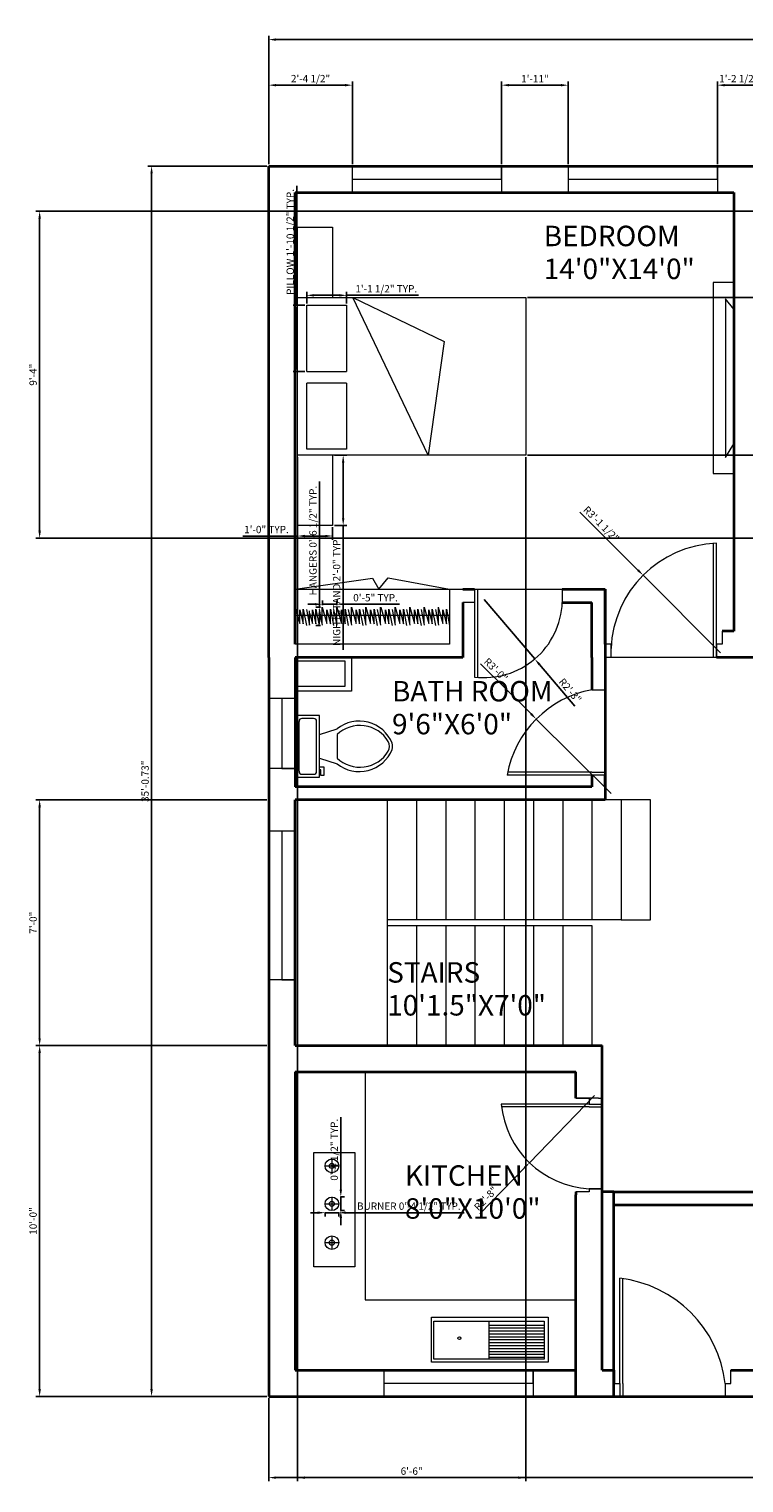
# Model space of a CAD drawing. Units: inches. Extents: x 1379 to 1989, y 1900 to 2397.
# Tile 1 of 3: x 1379 to 1623, y 1900 to 2397. Entities that reach past the tile are written whole.
import ezdxf

# ---------------------------------------------------------------- set-up
doc = ezdxf.new("R2010")
doc.units = ezdxf.units.IN
for name, color, linetype, lineweight in [('A-ANNO-DIMS', 2, 'Continuous', 18), ('A-AREA-IDEN', 7, 'Continuous', 18), ('A-DOOR', 3, 'Continuous', 18), ('A-EQPM', 9, 'Continuous', 18), ('A-FLOR-CASE', 9, 'Continuous', 18), ('A-FLOR-FIXT', 8, 'Continuous', 18), ('A-FLOR-FIXT-PATT', 8, 'Continuous', 13), ('A-FLOR-STRS', 7, 'Continuous', 18), ('A-FURN', 8, 'Continuous', 18), ('A-GLAZ', 4, 'Continuous', 18), ('A-WALL', 7, 'Continuous', 35)]:
    doc.layers.add(name, color=color, linetype=linetype, lineweight=lineweight)
doc.styles.get("Standard").update_dxf_attribs({"font": 'arial.ttf'})
doc.dimstyles.new('ISO-25', dxfattribs={"dimtxt": 2.5, "dimasz": 2.5, "dimexe": 1.25, "dimexo": 0.625, "dimtad": 1, "dimlunit": 3, "dimtxsty": 'Standard', "dimcen": 2.5, "dimadec": 0, "dimazin": 0, "dimtfac": 1, "dimtmove": 0, "dimatfit": 3, "dimfxl": 1, "dimarcsym": 0})

# ---------------------------------------------------------------- blocks, each defined once
blk = doc.blocks.new('*U2')
for p, q in [((9.5, -6), (9.5, -2)), ((-10, -8.5), (-8, -8.5)), ((-10, -9.5), (-10, -8.5)), ((-7, -9.5), (-10, -9.5)), ((-8, -8.5), (-8, -8)), ((-7, -8), (-7, -9.5)), ((-4, -8), (-6, -14)), ((4, -8), (6, -14)), ((4, -14), (-4, -14))]:
    blk.add_line(p, q)
blk.add_lwpolyline([(10.5, -8), (10.5, 0), (-10.5, 0), (-10.5, -8)], close=True)
for points in [[(-9.5, -2), (-9.5, -6)], [(8.5, -1), (-8.5, -1)], [(-8.5, -7), (8.5, -7)]]:
    blk.add_lwpolyline(points)
for centre, radius, start, end in [((-8.62, -1.88), 0.884, 81.8699, 188.1301), ((8.62, -1.88), 0.884, 351.8699, 98.1301), ((-8.62, -6.12), 0.884, 171.8699, 278.1301), ((8.62, -6.12), 0.884, 261.8699, 8.1301), ((3.52, -21.58), 12.17, 141.4691, 247.9714), ((4.2, -21.82), 11.33, 136.3677, 238.9468), ((-3.52, -21.58), 12.17, 292.0284, 38.5307), ((-4.2, -21.82), 11.33, 301.053, 43.6321), ((0, -27.88), 4, 245.7318, 294.2682), ((0, -29), 4, 254.8605, 285.1395)]:
    blk.add_arc(centre, radius, start, end)
blk = doc.blocks.new('*D6')
at = {"layer": 'A-ANNO-DIMS', "color": 0, "lineweight": -2, "transparency": 16777216}
for p, q in [((1460.41, 2350.93), (1460.41, 2394.79)), ((1462.91, 2393.54), (1912.41, 2393.54)), ((1914.91, 2350.93), (1914.91, 2394.79))]:
    blk.add_line(p, q, dxfattribs=at)
at = {"layer": 'A-ANNO-DIMS', "color": 0, "transparency": 16777216}
for points in [[(1462.91, 2393.95), (1462.91, 2393.12), (1460.41, 2393.54)], [(1912.41, 2393.95), (1912.41, 2393.12), (1914.91, 2393.54)]]:
    blk.add_solid(points, dxfattribs=at)
at = {"layer": 'Defpoints', "color": 0, "transparency": 16777216}
for p in [(1914.91, 2393.54), (1460.41, 2350.31), (1914.91, 2350.31)]:
    blk.add_point(p, dxfattribs=at)
at = {"layer": 'A-ANNO-DIMS', "color": 0, "transparency": 16777216, "insert": (1687.66, 2395.44), "char_height": 2.5, "attachment_point": 5}
blk.add_mtext('37\'-10.5"', dxfattribs=at)
blk = doc.blocks.new('*D7')
at = {"layer": 'A-ANNO-DIMS', "color": 0, "lineweight": -2, "transparency": 16777216}
for p, q in [((1459.79, 2350.31), (1419.13, 2350.31)), ((1420.38, 2347.81), (1420.38, 1932.08)), ((1459.79, 1929.58), (1419.13, 1929.58))]:
    blk.add_line(p, q, dxfattribs=at)
at = {"layer": 'A-ANNO-DIMS', "color": 0, "transparency": 16777216}
for points in [[(1419.96, 2347.81), (1420.79, 2347.81), (1420.38, 2350.31)], [(1419.96, 1932.08), (1420.79, 1932.08), (1420.38, 1929.58)]]:
    blk.add_solid(points, dxfattribs=at)
at = {"layer": 'Defpoints', "color": 0, "transparency": 16777216}
for p in [(1460.41, 2350.31), (1420.38, 1929.58), (1460.41, 1929.58)]:
    blk.add_point(p, dxfattribs=at)
at = {"layer": 'A-ANNO-DIMS', "color": 0, "transparency": 16777216, "insert": (1418.48, 2139.94), "char_height": 2.5, "attachment_point": 5, "rotation": 90}
blk.add_mtext('35\'-0.73"', dxfattribs=at)
blk = doc.blocks.new('WIN-51IN')
for p, q in [((0, 51), (9, 51)), ((4.5, 51), (4.5, 0)), ((9, 0), (0, 0)), ((4.5, 0), (9, 0))]:
    blk.add_line(p, q)
blk = doc.blocks.new('WIN-24IN')
for p, q in [((0, 24), (9, 24)), ((4.5, 24), (4.5, 0)), ((9, 0), (0, 0)), ((4.5, 0), (9, 0))]:
    blk.add_line(p, q)
blk = doc.blocks.new('COOKTOP-BURNER')
for p, q in [((0, 2.33), (4.67, 2.33)), ((2.33, 4.67), (2.33, 0))]:
    blk.add_line(p, q)
for radius in [2.33, 0.875]:
    blk.add_circle((2.33, 2.33), radius)
blk = doc.blocks.new('BED-PILLOW')
blk.add_line((0, 0), (13.66, 0))
blk.add_lwpolyline([(0, 0), (0, 22.6), (13.66, 22.6), (13.66, 0)])
blk = doc.blocks.new('CLOSET-GARMENT-CLUSTER')
for p, q in [((0, 6.34), (1.58, 0.7)), ((1.58, 0.7), (1.58, 5.41)), ((1.58, 5.41), (2.79, 0.56)), ((2.79, 0.56), (2.79, 5.59)), ((2.79, 5.59), (3.87, 0)), ((3.87, 5.45), (4.94, 0.19)), ((4.94, 0.83), (4.94, 6.28))]:
    blk.add_line(p, q)
blk = doc.blocks.new('CLOSET-GARMENT-CLUSTER-END')
for p, q in [((0, 5.45), (1.07, 0.19)), ((1.07, 0.19), (1.07, 5.08)), ((2.05, 0.7), (2.05, 5.41)), ((2.05, 5.41), (3.26, 0.56)), ((3.26, 0.56), (3.26, 5.59)), ((3.26, 5.59), (4.34, 0)), ((4.34, 5.45), (5.41, 0.19)), ((5.41, 0.83), (5.41, 6.28)), ((1.07, 0.83), (1.07, 4.19)), ((1.07, 4.19), (2.05, 0.7))]:
    blk.add_line(p, q)
blk = doc.blocks.new('BEDSIDE-TABLE-12X24')
for p, q in [((0, 0), (0, 24)), ((0, 24), (12, 24)), ((12, 24), (12, 0))]:
    blk.add_line(p, q)
blk = doc.blocks.new('*D19')
at = {"layer": 'A-ANNO-DIMS', "color": 0, "lineweight": -2, "transparency": 16777216}
for p, q in [((1470, 2302.71), (1470, 2343.51)), ((1472.76, 2302.71), (1468.75, 2302.71)), ((1470, 2282.61), (1470, 2300.21)), ((1472.76, 2280.11), (1468.75, 2280.11))]:
    blk.add_line(p, q, dxfattribs=at)
at = {"layer": 'A-ANNO-DIMS', "color": 0, "transparency": 16777216}
for points in [[(1469.58, 2300.21), (1470.42, 2300.21), (1470, 2302.71)], [(1469.58, 2282.61), (1470.42, 2282.61), (1470, 2280.11)]]:
    blk.add_solid(points, dxfattribs=at)
at = {"layer": 'Defpoints', "color": 0, "transparency": 16777216}
for p in [(1470, 2302.71), (1473.39, 2302.71), (1473.39, 2280.11)]:
    blk.add_point(p, dxfattribs=at)
at = {"layer": 'A-ANNO-DIMS', "color": 0, "transparency": 16777216, "insert": (1468.08, 2324.36), "char_height": 2.5, "attachment_point": 5, "rotation": 90}
blk.add_mtext('PILLOW 1\'-10 1/2" TYP.', dxfattribs=at)
blk = doc.blocks.new('*D20')
at = {"layer": 'A-ANNO-DIMS', "color": 0, "lineweight": -2, "transparency": 16777216}
for p, q in [((1473.39, 2303.34), (1473.39, 2307.35)), ((1487.05, 2303.34), (1487.05, 2307.35)), ((1475.89, 2306.1), (1484.55, 2306.1)), ((1487.05, 2306.1), (1511.63, 2306.1))]:
    blk.add_line(p, q, dxfattribs=at)
at = {"layer": 'A-ANNO-DIMS', "color": 0, "transparency": 16777216}
for points in [[(1475.89, 2306.52), (1475.89, 2305.68), (1473.39, 2306.1)], [(1484.55, 2306.52), (1484.55, 2305.68), (1487.05, 2306.1)]]:
    blk.add_solid(points, dxfattribs=at)
at = {"layer": 'Defpoints', "color": 0, "transparency": 16777216}
for p in [(1473.39, 2302.71), (1487.05, 2306.1), (1487.05, 2302.71)]:
    blk.add_point(p, dxfattribs=at)
at = {"layer": 'A-ANNO-DIMS', "color": 0, "transparency": 16777216, "insert": (1500.59, 2308.02), "char_height": 2.5, "attachment_point": 5}
blk.add_mtext('1\'-1 1/2" TYP.', dxfattribs=at)
blk = doc.blocks.new('*D21')
at = {"layer": 'A-ANNO-DIMS', "color": 0, "lineweight": -2, "transparency": 16777216}
for p, q in [((1482.89, 2251.4), (1487.12, 2251.4)), ((1485.87, 2248.9), (1485.87, 2229.9)), ((1482.89, 2227.4), (1487.12, 2227.4)), ((1485.87, 2227.4), (1485.87, 2184.86))]:
    blk.add_line(p, q, dxfattribs=at)
at = {"layer": 'A-ANNO-DIMS', "color": 0, "transparency": 16777216}
for points in [[(1485.45, 2248.9), (1486.28, 2248.9), (1485.87, 2251.4)], [(1485.45, 2229.9), (1486.28, 2229.9), (1485.87, 2227.4)]]:
    blk.add_solid(points, dxfattribs=at)
at = {"layer": 'Defpoints', "color": 0, "transparency": 16777216}
for p in [(1482.27, 2251.4), (1482.27, 2227.4), (1485.87, 2227.4)]:
    blk.add_point(p, dxfattribs=at)
at = {"layer": 'A-ANNO-DIMS', "color": 0, "transparency": 16777216, "insert": (1483.95, 2204.88), "char_height": 2.5, "attachment_point": 5, "rotation": 90}
blk.add_mtext('NIGHTSTAND 2\'-0" TYP.', dxfattribs=at)
blk = doc.blocks.new('*D22')
at = {"layer": 'A-ANNO-DIMS', "color": 0, "lineweight": -2, "transparency": 16777216}
for p, q in [((1470.27, 2223.8), (1451.51, 2223.8)), ((1470.27, 2226.77), (1470.27, 2222.55)), ((1479.77, 2223.8), (1472.77, 2223.8)), ((1482.27, 2226.77), (1482.27, 2222.55))]:
    blk.add_line(p, q, dxfattribs=at)
at = {"layer": 'A-ANNO-DIMS', "color": 0, "transparency": 16777216}
for points in [[(1472.77, 2224.21), (1472.77, 2223.38), (1470.27, 2223.8)], [(1479.77, 2224.21), (1479.77, 2223.38), (1482.27, 2223.8)]]:
    blk.add_solid(points, dxfattribs=at)
at = {"layer": 'Defpoints', "color": 0, "transparency": 16777216}
for p in [(1470.27, 2227.4), (1482.27, 2227.4), (1470.27, 2223.8)]:
    blk.add_point(p, dxfattribs=at)
at = {"layer": 'A-ANNO-DIMS', "color": 0, "transparency": 16777216, "insert": (1459.64, 2225.7), "char_height": 2.5, "attachment_point": 5}
blk.add_mtext('1\'-0" TYP.', dxfattribs=at)
blk = doc.blocks.new('*D23')
at = {"layer": 'A-ANNO-DIMS', "color": 0, "lineweight": -2, "transparency": 16777216}
for p, q in [((1477.19, 1992.42), (1474.69, 1992.42)), ((1479.69, 1992.5), (1479.69, 1991.17)), ((1479.69, 1992.42), (1484.35, 1992.42)), ((1484.35, 1992.5), (1484.35, 1991.17)), ((1486.85, 1992.42), (1527.27, 1992.42))]:
    blk.add_line(p, q, dxfattribs=at)
at = {"layer": 'A-ANNO-DIMS', "color": 0, "transparency": 16777216}
for points in [[(1477.19, 1992.84), (1477.19, 1992), (1479.69, 1992.42)], [(1486.85, 1992.84), (1486.85, 1992), (1484.35, 1992.42)]]:
    blk.add_solid(points, dxfattribs=at)
at = {"layer": 'Defpoints', "color": 0, "transparency": 16777216}
for p in [(1479.69, 1993.12), (1484.35, 1993.12), (1484.35, 1992.42)]:
    blk.add_point(p, dxfattribs=at)
at = {"layer": 'A-ANNO-DIMS', "color": 0, "transparency": 16777216, "insert": (1508.31, 1994.34), "char_height": 2.5, "attachment_point": 5}
blk.add_mtext('BURNER 0\'-4 1/2" TYP.', dxfattribs=at)
blk = doc.blocks.new('*D24')
at = {"layer": 'A-ANNO-DIMS', "color": 0, "lineweight": -2, "transparency": 16777216}
for p, q in [((1485.05, 2000.29), (1485.05, 2025.1)), ((1484.98, 1997.79), (1486.3, 1997.79)), ((1485.05, 1993.12), (1485.05, 1997.79)), ((1484.98, 1993.12), (1486.3, 1993.12)), ((1485.05, 1990.62), (1485.05, 1988.12))]:
    blk.add_line(p, q, dxfattribs=at)
at = {"layer": 'A-ANNO-DIMS', "color": 0, "transparency": 16777216}
for points in [[(1484.64, 2000.29), (1485.47, 2000.29), (1485.05, 1997.79)], [(1484.64, 1990.62), (1485.47, 1990.62), (1485.05, 1993.12)]]:
    blk.add_solid(points, dxfattribs=at)
at = {"layer": 'Defpoints', "color": 0, "transparency": 16777216}
for p in [(1484.35, 1997.79), (1485.05, 1997.79), (1484.35, 1993.12)]:
    blk.add_point(p, dxfattribs=at)
at = {"layer": 'A-ANNO-DIMS', "color": 0, "transparency": 16777216, "insert": (1483.14, 2013.94), "char_height": 2.5, "attachment_point": 5, "rotation": 90}
blk.add_mtext('0\'-4 1/2" TYP.', dxfattribs=at)
blk = doc.blocks.new('*D25')
at = {"layer": 'A-ANNO-DIMS', "color": 0, "lineweight": -2, "transparency": 16777216}
for p, q in [((1477.79, 2199.52), (1477.79, 2242.44)), ((1478.11, 2199.52), (1476.54, 2199.52)), ((1478.11, 2193.18), (1476.54, 2193.18)), ((1477.79, 2195.68), (1477.79, 2197.02))]:
    blk.add_line(p, q, dxfattribs=at)
at = {"layer": 'A-ANNO-DIMS', "color": 0, "transparency": 16777216}
for points in [[(1477.37, 2197.02), (1478.2, 2197.02), (1477.79, 2199.52)], [(1477.37, 2195.68), (1478.2, 2195.68), (1477.79, 2193.18)]]:
    blk.add_solid(points, dxfattribs=at)
at = {"layer": 'Defpoints', "color": 0, "transparency": 16777216}
for p in [(1477.79, 2199.52), (1478.74, 2199.52), (1478.74, 2193.18)]:
    blk.add_point(p, dxfattribs=at)
at = {"layer": 'A-ANNO-DIMS', "color": 0, "transparency": 16777216, "insert": (1475.87, 2222.23), "char_height": 2.5, "attachment_point": 5, "rotation": 90}
blk.add_mtext('HANGERS 0\'-6 1/2" TYP.', dxfattribs=at)
blk = doc.blocks.new('*D26')
at = {"layer": 'A-ANNO-DIMS', "color": 0, "lineweight": -2, "transparency": 16777216}
for p, q in [((1476.24, 2200.47), (1473.74, 2200.47)), ((1478.74, 2200.14), (1478.74, 2201.72)), ((1478.74, 2200.47), (1483.68, 2200.47)), ((1483.68, 2200.14), (1483.68, 2201.72)), ((1486.18, 2200.47), (1505.17, 2200.47))]:
    blk.add_line(p, q, dxfattribs=at)
at = {"layer": 'A-ANNO-DIMS', "color": 0, "transparency": 16777216}
for points in [[(1476.24, 2200.88), (1476.24, 2200.05), (1478.74, 2200.47)], [(1486.18, 2200.88), (1486.18, 2200.05), (1483.68, 2200.47)]]:
    blk.add_solid(points, dxfattribs=at)
at = {"layer": 'Defpoints', "color": 0, "transparency": 16777216}
for p in [(1478.74, 2199.52), (1483.68, 2200.47), (1483.68, 2199.52)]:
    blk.add_point(p, dxfattribs=at)
at = {"layer": 'A-ANNO-DIMS', "color": 0, "transparency": 16777216, "insert": (1496.92, 2202.37), "char_height": 2.5, "attachment_point": 5}
blk.add_mtext('0\'-5" TYP.', dxfattribs=at)
blk = doc.blocks.new('*D29')
at = {"layer": 'A-ANNO-DIMS', "color": 0, "lineweight": -2, "transparency": 16777216}
for p, q in [((1959.91, 1941.48), (1959.91, 1900.58)), ((1460.41, 1928.96), (1460.41, 1900.58)), ((1462.91, 1901.83), (1957.41, 1901.83))]:
    blk.add_line(p, q, dxfattribs=at)
at = {"layer": 'A-ANNO-DIMS', "color": 0, "transparency": 16777216}
for points in [[(1462.91, 1902.24), (1462.91, 1901.41), (1460.41, 1901.83)], [(1957.41, 1902.24), (1957.41, 1901.41), (1959.91, 1901.83)]]:
    blk.add_solid(points, dxfattribs=at)
at = {"layer": 'Defpoints', "color": 0, "transparency": 16777216}
for p in [(1959.91, 1942.11), (1460.41, 1929.58), (1959.91, 1901.83)]:
    blk.add_point(p, dxfattribs=at)
at = {"layer": 'A-ANNO-DIMS', "color": 0, "transparency": 16777216, "insert": (1710.16, 1903.75), "char_height": 2.5, "attachment_point": 5}
blk.add_mtext('41\'-7 1/2"', dxfattribs=at)
blk = doc.blocks.new('*D33')
at = {"layer": 'A-ANNO-DIMS', "color": 0, "lineweight": -2, "transparency": 16777216}
for p, q in [((1460.41, 2350.93), (1460.41, 2379.21)), ((1462.91, 2377.96), (1486.52, 2377.96)), ((1489.02, 2350.93), (1489.02, 2379.21))]:
    blk.add_line(p, q, dxfattribs=at)
at = {"layer": 'A-ANNO-DIMS', "color": 0, "transparency": 16777216}
for points in [[(1462.91, 2378.37), (1462.91, 2377.54), (1460.41, 2377.96)], [(1486.52, 2378.37), (1486.52, 2377.54), (1489.02, 2377.96)]]:
    blk.add_solid(points, dxfattribs=at)
at = {"layer": 'Defpoints', "color": 0, "transparency": 16777216}
for p in [(1489.02, 2377.96), (1460.41, 2350.31), (1489.02, 2350.31)]:
    blk.add_point(p, dxfattribs=at)
at = {"layer": 'A-ANNO-DIMS', "color": 0, "transparency": 16777216, "insert": (1474.71, 2379.88), "char_height": 2.5, "attachment_point": 5}
blk.add_mtext('2\'-4 1/2"', dxfattribs=at)
blk = doc.blocks.new('*D34')
at = {"layer": 'A-ANNO-DIMS', "color": 0, "lineweight": -2, "transparency": 16777216}
for p, q in [((1540.02, 2350.93), (1540.02, 2379.21)), ((1542.52, 2377.96), (1560.28, 2377.96)), ((1562.78, 2350.93), (1562.78, 2379.21))]:
    blk.add_line(p, q, dxfattribs=at)
at = {"layer": 'A-ANNO-DIMS', "color": 0, "transparency": 16777216}
for points in [[(1542.52, 2378.37), (1542.52, 2377.54), (1540.02, 2377.96)], [(1560.28, 2378.37), (1560.28, 2377.54), (1562.78, 2377.96)]]:
    blk.add_solid(points, dxfattribs=at)
at = {"layer": 'Defpoints', "color": 0, "transparency": 16777216}
for p in [(1562.78, 2377.96), (1540.02, 2350.31), (1562.78, 2350.31)]:
    blk.add_point(p, dxfattribs=at)
at = {"layer": 'A-ANNO-DIMS', "color": 0, "transparency": 16777216, "insert": (1551.4, 2379.84), "char_height": 2.5, "attachment_point": 5}
blk.add_mtext('1\'-11"', dxfattribs=at)
blk = doc.blocks.new('*D35')
at = {"layer": 'A-ANNO-DIMS', "color": 0, "lineweight": -2, "transparency": 16777216}
for p, q in [((1613.78, 2350.93), (1613.78, 2379.21)), ((1616.28, 2377.96), (1625.91, 2377.96)), ((1628.41, 2350.93), (1628.41, 2379.21))]:
    blk.add_line(p, q, dxfattribs=at)
at = {"layer": 'A-ANNO-DIMS', "color": 0, "transparency": 16777216}
for points in [[(1616.28, 2378.37), (1616.28, 2377.54), (1613.78, 2377.96)], [(1625.91, 2378.37), (1625.91, 2377.54), (1628.41, 2377.96)]]:
    blk.add_solid(points, dxfattribs=at)
at = {"layer": 'Defpoints', "color": 0, "transparency": 16777216}
for p in [(1628.41, 2377.96), (1613.78, 2350.31), (1628.41, 2350.31)]:
    blk.add_point(p, dxfattribs=at)
at = {"layer": 'A-ANNO-DIMS', "color": 0, "transparency": 16777216, "insert": (1621.1, 2379.88), "char_height": 2.5, "attachment_point": 5}
blk.add_mtext('1\'-2 1/2"', dxfattribs=at)
blk = doc.blocks.new('*D38')
at = {"layer": 'A-ANNO-DIMS', "color": 0, "lineweight": -2, "transparency": 16777216}
for p, q in [((1459.79, 2049.58), (1380.86, 2049.58)), ((1382.11, 1932.08), (1382.11, 2047.08)), ((1459.79, 1929.58), (1380.86, 1929.58))]:
    blk.add_line(p, q, dxfattribs=at)
at = {"layer": 'A-ANNO-DIMS', "color": 0, "transparency": 16777216}
for points in [[(1381.7, 2047.08), (1382.53, 2047.08), (1382.11, 2049.58)], [(1381.7, 1932.08), (1382.53, 1932.08), (1382.11, 1929.58)]]:
    blk.add_solid(points, dxfattribs=at)
at = {"layer": 'Defpoints', "color": 0, "transparency": 16777216}
for p in [(1382.11, 2049.58), (1460.41, 2049.58), (1460.41, 1929.58)]:
    blk.add_point(p, dxfattribs=at)
at = {"layer": 'A-ANNO-DIMS', "color": 0, "transparency": 16777216, "insert": (1380.21, 1989.58), "char_height": 2.5, "attachment_point": 5, "rotation": 90}
blk.add_mtext('10\'-0"', dxfattribs=at)
blk = doc.blocks.new('*D39')
at = {"layer": 'A-ANNO-DIMS', "color": 0, "lineweight": -2, "transparency": 16777216}
for p, q in [((1459.79, 2133.58), (1380.86, 2133.58)), ((1382.11, 2052.08), (1382.11, 2131.08)), ((1459.79, 2049.58), (1380.86, 2049.58))]:
    blk.add_line(p, q, dxfattribs=at)
at = {"layer": 'A-ANNO-DIMS', "color": 0, "transparency": 16777216}
for points in [[(1381.7, 2131.08), (1382.53, 2131.08), (1382.11, 2133.58)], [(1381.7, 2052.08), (1382.53, 2052.08), (1382.11, 2049.58)]]:
    blk.add_solid(points, dxfattribs=at)
at = {"layer": 'Defpoints', "color": 0, "transparency": 16777216}
for p in [(1382.11, 2133.58), (1460.41, 2133.58), (1460.41, 2049.58)]:
    blk.add_point(p, dxfattribs=at)
at = {"layer": 'A-ANNO-DIMS', "color": 0, "transparency": 16777216, "insert": (1380.21, 2091.58), "char_height": 2.5, "attachment_point": 5, "rotation": 90}
blk.add_mtext('7\'-0"', dxfattribs=at)
blk = doc.blocks.new('*D40')
at = {"layer": 'A-ANNO-DIMS', "color": 0, "lineweight": -2, "transparency": 16777216}
for p, q in [((1470.27, 2250.77), (1470.27, 1900.58)), ((1548.27, 2250.77), (1548.27, 1900.58)), ((1472.77, 1901.83), (1545.77, 1901.83))]:
    blk.add_line(p, q, dxfattribs=at)
at = {"layer": 'A-ANNO-DIMS', "color": 0, "transparency": 16777216}
for points in [[(1472.77, 1902.24), (1472.77, 1901.41), (1470.27, 1901.83)], [(1545.77, 1902.24), (1545.77, 1901.41), (1548.27, 1901.83)]]:
    blk.add_solid(points, dxfattribs=at)
at = {"layer": 'Defpoints', "color": 0, "transparency": 16777216}
for p in [(1470.27, 2251.4), (1548.27, 2251.4), (1548.27, 1901.83)]:
    blk.add_point(p, dxfattribs=at)
at = {"layer": 'A-ANNO-DIMS', "color": 0, "transparency": 16777216, "insert": (1509.27, 1903.73), "char_height": 2.5, "attachment_point": 5}
blk.add_mtext('6\'-6"', dxfattribs=at)
blk = doc.blocks.new('*D41')
at = {"layer": 'A-ANNO-DIMS', "color": 0, "lineweight": -2, "transparency": 16777216}
for p, q in [((1548.89, 2305.4), (1988.81, 2305.4)), ((1987.56, 2302.9), (1987.56, 2253.9)), ((1548.89, 2251.4), (1988.81, 2251.4))]:
    blk.add_line(p, q, dxfattribs=at)
at = {"layer": 'A-ANNO-DIMS', "color": 0, "transparency": 16777216}
for points in [[(1987.14, 2302.9), (1987.98, 2302.9), (1987.56, 2305.4)], [(1987.14, 2253.9), (1987.98, 2253.9), (1987.56, 2251.4)]]:
    blk.add_solid(points, dxfattribs=at)
at = {"layer": 'Defpoints', "color": 0, "transparency": 16777216}
for p in [(1548.27, 2305.4), (1548.27, 2251.4), (1987.56, 2251.4)]:
    blk.add_point(p, dxfattribs=at)
at = {"layer": 'A-ANNO-DIMS', "color": 0, "transparency": 16777216, "insert": (1985.66, 2278.4), "char_height": 2.5, "attachment_point": 5, "rotation": 90}
blk.add_mtext('4\'-6"', dxfattribs=at)
blk = doc.blocks.new('*D43')
at = {"layer": 'A-ANNO-DIMS', "color": 0, "lineweight": -2, "transparency": 16777216}
for p, q in [((1811.35, 2334.84), (1380.86, 2334.84)), ((1382.11, 2332.34), (1382.11, 2225.59)), ((1875.73, 2223.09), (1380.86, 2223.09))]:
    blk.add_line(p, q, dxfattribs=at)
at = {"layer": 'A-ANNO-DIMS', "color": 0, "transparency": 16777216}
for points in [[(1381.7, 2332.34), (1382.53, 2332.34), (1382.11, 2334.84)], [(1381.7, 2225.59), (1382.53, 2225.59), (1382.11, 2223.09)]]:
    blk.add_solid(points, dxfattribs=at)
at = {"layer": 'Defpoints', "color": 0, "transparency": 16777216}
for p in [(1811.97, 2334.84), (1382.11, 2223.09), (1876.36, 2223.09)]:
    blk.add_point(p, dxfattribs=at)
at = {"layer": 'A-ANNO-DIMS', "color": 0, "transparency": 16777216, "insert": (1380.21, 2278.96), "char_height": 2.5, "attachment_point": 5, "rotation": 90}
blk.add_mtext('9\'-4"', dxfattribs=at)
blk = doc.blocks.new('*D46')
at = {"layer": 'A-ANNO-DIMS', "color": 0, "lineweight": -2, "transparency": 16777216}
for p, q in [((1566.8, 2232), (1586.62, 2212.15)), ((1614.88, 2183.84), (1588.38, 2210.38))]:
    blk.add_line(p, q, dxfattribs=at)
at = {"layer": 'A-ANNO-DIMS', "color": 0, "transparency": 16777216}
blk.add_solid([(1586.91, 2212.44), (1586.32, 2211.85), (1588.38, 2210.38)], dxfattribs=at)
at = {"layer": 'Defpoints', "color": 0, "transparency": 16777216}
for p in [(1588.38, 2210.38), (1614.88, 2183.84)]:
    blk.add_point(p, dxfattribs=at)
at = {"layer": 'A-ANNO-DIMS', "color": 0, "transparency": 16777216, "insert": (1573.85, 2227.65), "char_height": 2.5, "attachment_point": 5, "rotation": 314.9518}
blk.add_mtext('R3\'-1 1/2"', dxfattribs=at)
blk = doc.blocks.new('*D47')
at = {"layer": 'A-ANNO-DIMS', "color": 0, "lineweight": -2, "transparency": 16777216}
for p, q in [((1532.83, 2180.11), (1550.08, 2162.96)), ((1577.48, 2135.72), (1551.85, 2161.2))]:
    blk.add_line(p, q, dxfattribs=at)
at = {"layer": 'A-ANNO-DIMS', "color": 0, "transparency": 16777216}
blk.add_solid([(1550.37, 2163.26), (1549.79, 2162.67), (1551.85, 2161.2)], dxfattribs=at)
at = {"layer": 'Defpoints', "color": 0, "transparency": 16777216}
for p in [(1551.85, 2161.2), (1577.48, 2135.72)]:
    blk.add_point(p, dxfattribs=at)
at = {"layer": 'A-ANNO-DIMS', "color": 0, "transparency": 16777216, "insert": (1537.82, 2177.83), "char_height": 2.5, "attachment_point": 5, "rotation": 315.173}
blk.add_mtext('R3\'-0"', dxfattribs=at)
blk = doc.blocks.new('*D48')
at = {"layer": 'A-ANNO-DIMS', "color": 0, "lineweight": -2, "transparency": 16777216}
for p, q in [((1571.77, 2032.52), (1549.53, 2009.52)), ((1532.61, 1992.02), (1547.79, 2007.72))]:
    blk.add_line(p, q, dxfattribs=at)
at = {"layer": 'A-ANNO-DIMS', "color": 0, "transparency": 16777216}
blk.add_solid([(1547.5, 2008.01), (1548.09, 2007.43), (1549.53, 2009.52)], dxfattribs=at)
at = {"layer": 'Defpoints', "color": 0, "transparency": 16777216}
for p in [(1571.77, 2032.52), (1549.53, 2009.52)]:
    blk.add_point(p, dxfattribs=at)
at = {"layer": 'A-ANNO-DIMS', "color": 0, "transparency": 16777216, "insert": (1534.82, 1997.04), "char_height": 2.5, "attachment_point": 5, "rotation": 45.9708}
blk.add_mtext('R2\'-8"', dxfattribs=at)
blk = doc.blocks.new('*D49')
at = {"layer": 'A-ANNO-DIMS', "color": 0, "lineweight": -2, "transparency": 16777216}
for p, q in [((1534.02, 2202.14), (1551.35, 2181.75)), ((1565.08, 2165.6), (1552.97, 2179.85))]:
    blk.add_line(p, q, dxfattribs=at)
at = {"layer": 'A-ANNO-DIMS', "color": 0, "transparency": 16777216}
blk.add_solid([(1553.28, 2180.12), (1552.65, 2179.58), (1551.35, 2181.75)], dxfattribs=at)
at = {"layer": 'Defpoints', "color": 0, "transparency": 16777216}
for p in [(1534.02, 2202.14), (1551.35, 2181.75)]:
    blk.add_point(p, dxfattribs=at)
at = {"layer": 'A-ANNO-DIMS', "color": 0, "transparency": 16777216, "insert": (1563.19, 2170.75), "char_height": 2.5, "attachment_point": 5, "rotation": 310.3656}
blk.add_mtext('R2\'-3"', dxfattribs=at)

msp = doc.modelspace()

# ---------------------------------------------------------------- hatches: boundary and pattern name
at = {"layer": 'A-FLOR-FIXT-PATT'}
h = msp.add_hatch(dxfattribs=at)
h.set_pattern_fill('ANSI31', color=256, scale=0.314961, angle=-45, style=0)
h.paths.add_polyline_path([(1535.728, 1942.741), (1554.59, 1942.741), (1554.59, 1954.741), (1535.728, 1954.741)])

# ---------------------------------------------------------------- linework, layer by layer
at = {"layer": 'A-DOOR'}
for p, q in [((1612.41, 2185.308), (1612.41, 2221.255)), ((1613.41, 2185.308), (1613.41, 2221.308)), ((1530.753, 2205.582), (1530.753, 2201.082)), ((1530.753, 2205.582), (1560.753, 2205.582)), ((1530.753, 2205.582), (1530.753, 2175.582)), ((1531.753, 2205.582), (1531.753, 2175.582)), ((1560.753, 2205.582), (1560.753, 2201.082)), ((1530.753, 2201.082), (1526.753, 2201.082)), ((1619.41, 2191.308), (1615.41, 2191.308)), ((1615.41, 2191.308), (1615.41, 2186.808)), ((1577.41, 2186.808), (1575.41, 2186.808)), ((1577.41, 2182.308), (1577.41, 2186.808)), ((1612.41, 2182.308), (1612.41, 2185.308)), ((1615.41, 2186.808), (1613.41, 2186.808)), ((1613.41, 2186.808), (1613.41, 2182.308)), ((1615.41, 2186.808), (1613.41, 2186.808)), ((1613.41, 2182.308), (1613.41, 2185.308)), ((1577.41, 2182.308), (1575.41, 2182.308)), ((1613.41, 2182.308), (1577.41, 2182.308)), ((1575.41, 2171.082), (1570.91, 2171.082)), ((1575.41, 2142.082), (1575.41, 2171.082)), ((1570.91, 2143.082), (1542.104, 2143.082)), ((1570.91, 2143.082), (1575.41, 2143.082)), ((1570.91, 2142.082), (1541.91, 2142.082)), ((1575.41, 2142.082), (1570.91, 2142.082)), ((1569.91, 2029.582), (1539.91, 2029.582)), ((1569.91, 2028.582), (1539.91, 2028.582)), ((1573.101, 2031.582), (1565.41, 2031.582)), ((1565.41, 2031.582), (1569.91, 2031.582)), ((1569.91, 2031.582), (1569.91, 2029.582)), ((1569.91, 2029.582), (1574.41, 2029.582)), ((1569.91, 2028.582), (1574.41, 2028.582)), ((1573.101, 2031.582), (1574.41, 2031.582)), ((1569.91, 1999.582), (1565.41, 1999.582)), ((1569.91, 2000.582), (1574.41, 2000.582)), ((1574.41, 2000.582), (1569.91, 2000.582)), ((1574.41, 2000.582), (1569.91, 2000.582)), ((1569.91, 2000.582), (1569.91, 1999.582)), ((1569.91, 1998.582), (1569.91, 1998.582)), ((1580.41, 1933.978), (1580.41, 1969.978)), ((1581.41, 1933.978), (1581.41, 1969.851)), ((1578.41, 1933.978), (1580.41, 1933.978)), ((1580.41, 1933.978), (1580.41, 1929.582)), ((1581.41, 1933.978), (1581.41, 1929.582)), ((1616.41, 1933.978), (1616.41, 1929.582)), ((1616.41, 1933.978), (1618.41, 1933.978)), ((1618.41, 1933.978), (1618.41, 1938.582))]:
    msp.add_line(p, q, dxfattribs=at)
for centre, radius, start, end in [((1614.877, 2183.838), 37.498, 92.24183, 177.66061), ((1534.019, 2202.136), 26.755, 262.98798, 357.7411), ((1577.485, 2135.723), 36.138, 100.48207, 169.86542), ((1571.769, 2032.522), 31.994, 185.27318, 266.66886), ((1575.755, 1929.322), 40.921, 6.53202, 83.46798)]:
    msp.add_arc(centre, radius, start, end, dxfattribs=at)
at = {"layer": 'A-EQPM'}
msp.add_lwpolyline([(1475.816, 2012.99), (1489.79, 2012.99), (1489.79, 1973.888), (1475.816, 1973.888)], close=True, dxfattribs=at)
at = {"layer": 'A-FLOR-CASE'}
for p, q in [((1469.41, 2205.582), (1495.864, 2209.393)), ((1495.864, 2209.393), (1498.082, 2205.582)), ((1498.082, 2205.582), (1501.217, 2209.468)), ((1501.217, 2209.468), (1522.253, 2205.582)), ((1469.41, 2205.582), (1526.753, 2205.582)), ((1522.253, 2205.582), (1522.253, 2186.808)), ((1469.41, 2199.516), (1470.993, 2193.877)), ((1470.993, 2193.877), (1470.993, 2198.584)), ((1470.993, 2198.584), (1472.205, 2193.737)), ((1472.205, 2193.737), (1472.205, 2198.77)), ((1472.205, 2198.77), (1473.278, 2193.178)), ((1518.339, 2199.516), (1519.921, 2193.877)), ((1519.921, 2193.877), (1519.921, 2198.584)), ((1519.921, 2198.584), (1521.134, 2193.737)), ((1521.134, 2193.737), (1521.134, 2198.77)), ((1521.134, 2198.77), (1522.206, 2193.178)), ((1522.206, 2198.63), (1522.253, 2198.401)), ((1469.41, 2196.735), (1522.253, 2196.735)), ((1522.253, 2186.808), (1469.41, 2186.808)), ((1469.41, 2040.582), (1493.41, 2040.582)), ((1493.41, 2040.582), (1493.41, 1962.582)), ((1469.41, 1938.582), (1469.41, 1962.582)), ((1493.41, 1962.582), (1565.41, 1962.582))]:
    msp.add_line(p, q, dxfattribs=at)
at = {"layer": 'A-FLOR-FIXT'}
for p, q in [((1469.41, 2181.084), (1486.48, 2181.084)), ((1486.48, 2182.308), (1488.751, 2182.308)), ((1486.48, 2181.084), (1486.48, 2172.322)), ((1488.751, 2182.308), (1488.751, 2170.738)), ((1486.48, 2172.322), (1469.41, 2172.322)), ((1535.728, 1942.369), (1535.728, 1955.283))]:
    msp.add_line(p, q, dxfattribs=at)
msp.add_lwpolyline([(1488.751, 2170.738), (1469.41, 2170.738)], dxfattribs=at)
for points in [[(1516.053, 1956.745), (1555.93, 1956.745), (1555.93, 1941.32), (1516.053, 1941.32)], [(1516.866, 1955.283), (1554.59, 1955.283), (1554.59, 1942.369), (1516.866, 1942.369)]]:
    msp.add_lwpolyline(points, close=True, dxfattribs=at)
msp.add_circle((1525.572, 1949.528), 0.499, dxfattribs=at)
at = {"layer": 'A-FLOR-STRS'}
for p, q in [((1500.91, 2133.582), (1500.91, 2092.582)), ((1510.91, 2133.582), (1510.91, 2092.582)), ((1520.91, 2133.582), (1520.91, 2092.582)), ((1530.91, 2133.582), (1530.91, 2092.582)), ((1540.91, 2133.582), (1540.91, 2092.582)), ((1550.91, 2133.582), (1550.91, 2092.582)), ((1560.91, 2133.582), (1560.91, 2092.582)), ((1590.91, 2133.582), (1570.91, 2133.582)), ((1570.91, 2133.582), (1570.91, 2092.582)), ((1590.91, 2133.582), (1580.91, 2133.582)), ((1580.91, 2133.582), (1580.91, 2092.582)), ((1590.91, 2092.582), (1590.91, 2133.582)), ((1580.91, 2092.582), (1500.91, 2092.582)), ((1500.91, 2092.582), (1500.91, 2049.582)), ((1500.91, 2090.582), (1560.91, 2090.582)), ((1510.91, 2090.582), (1510.91, 2049.582)), ((1520.91, 2090.582), (1520.91, 2049.582)), ((1530.91, 2090.582), (1530.91, 2049.582)), ((1540.91, 2090.582), (1540.91, 2049.582)), ((1550.91, 2090.582), (1550.91, 2049.582)), ((1560.91, 2090.582), (1560.91, 2049.582)), ((1560.91, 2090.582), (1570.91, 2090.582)), ((1570.91, 2090.582), (1570.91, 2049.582)), ((1580.91, 2092.582), (1590.91, 2092.582))]:
    msp.add_line(p, q, dxfattribs=at)
at = {"layer": 'A-FURN'}
for p, q in [((1619.41, 2310.458), (1612.278, 2310.458)), ((1612.278, 2310.458), (1612.278, 2245.161)), ((1470.266, 2251.398), (1470.266, 2305.398)), ((1470.266, 2305.398), (1548.266, 2305.398)), ((1514.883, 2251.398), (1489.219, 2305.398)), ((1489.219, 2305.398), (1520.343, 2290.26)), ((1548.266, 2305.398), (1548.266, 2251.398)), ((1619.41, 2301.386), (1616.525, 2304.884)), ((1616.525, 2304.884), (1616.525, 2250.67)), ((1520.343, 2290.26), (1514.883, 2251.398)), ((1616.525, 2250.67), (1619.41, 2255.333)), ((1548.266, 2251.398), (1470.266, 2251.398)), ((1612.278, 2245.161), (1619.41, 2245.161))]:
    msp.add_line(p, q, dxfattribs=at)
at = {"layer": 'A-GLAZ'}
for p, q in [((1562.78, 2350.308), (1562.78, 2341.308)), ((1489.017, 2341.308), (1489.017, 2345.808))]:
    msp.add_line(p, q, dxfattribs=at)
msp.add_lwpolyline([(1562.78, 2345.808), (1613.78, 2345.808), (1613.78, 2350.308), (1613.78, 2341.308)], dxfattribs=at)
at = {"layer": 'A-WALL'}
for p, q in [((1460.41, 2350.308), (1628.41, 2350.308)), ((1460.41, 2182.308), (1460.41, 2350.308)), ((1469.41, 2341.308), (1619.41, 2341.308)), ((1469.41, 2186.808), (1469.41, 2341.308)), ((1619.41, 2341.308), (1619.41, 2191.308)), ((1526.753, 2205.582), (1530.753, 2205.582)), ((1560.753, 2205.582), (1570.91, 2205.582)), ((1570.91, 2205.582), (1575.41, 2205.582)), ((1575.41, 2186.808), (1575.41, 2205.582)), ((1575.41, 2205.582), (1575.41, 2133.582)), ((1526.753, 2201.082), (1526.753, 2182.308)), ((1560.753, 2201.082), (1570.91, 2201.082)), ((1570.91, 2182.308), (1570.91, 2201.082)), ((1619.41, 2191.308), (1615.41, 2191.308)), ((1460.41, 2182.308), (1460.41, 2133.582)), ((1526.753, 2182.308), (1469.41, 2182.308)), ((1469.41, 2182.308), (1469.41, 2138.082)), ((1570.91, 2182.308), (1570.91, 2171.082)), ((1628.41, 2182.308), (1613.41, 2182.308)), ((1570.91, 2138.082), (1469.41, 2138.082)), ((1570.91, 2142.082), (1570.91, 2138.082)), ((1575.41, 2138.082), (1575.41, 2142.082)), ((1460.41, 2133.582), (1460.41, 2049.582)), ((1575.41, 2133.582), (1469.41, 2133.582)), ((1469.41, 2049.582), (1469.41, 2133.582)), ((1460.41, 2049.582), (1460.41, 1929.582)), ((1469.41, 2049.582), (1565.41, 2049.582)), ((1565.41, 2049.582), (1574.385, 2049.582)), ((1574.385, 2049.582), (1574.41, 2049.582)), ((1574.41, 2040.582), (1574.41, 2049.582)), ((1469.41, 2040.582), (1469.41, 1938.582)), ((1469.41, 2040.582), (1565.41, 2040.582)), ((1565.41, 2031.582), (1565.41, 2040.582)), ((1574.41, 1938.582), (1574.41, 2040.582)), ((1574.41, 1938.582), (1574.41, 2008.582)), ((1565.41, 1999.582), (1565.41, 1998.582)), ((1565.41, 1929.582), (1565.41, 1998.582)), ((1578.41, 1999.582), (1574.41, 1999.582)), ((1578.41, 1929.582), (1578.41, 1999.582)), ((1578.41, 1999.582), (1639.91, 1999.582)), ((1578.41, 1995.082), (1695.41, 1995.082)), ((1469.41, 1938.582), (1565.41, 1938.582)), ((1574.41, 1938.582), (1578.41, 1938.582)), ((1578.41, 1938.582), (1578.41, 1933.978)), ((1618.41, 1938.582), (1770.91, 1938.582)), ((1460.41, 1929.582), (1469.41, 1929.582)), ((1469.41, 1929.582), (1565.41, 1929.582)), ((1565.41, 1929.582), (1744.577, 1929.582)), ((1578.41, 1929.478), (1578.41, 1929.582)), ((1578.41, 1929.582), (1578.41, 1929.478))]:
    msp.add_line(p, q, dxfattribs=at)

# ---------------------------------------------------------------- block references
at = {"layer": 'A-EQPM'}
for p in [(1479.686, 2006.102), (1479.686, 1993.12), (1479.686, 1979.845)]:
    msp.add_blockref('COOKTOP-BURNER', p, dxfattribs=at)
at = {"layer": 'A-FLOR-CASE'}
for name, p in [('CLOSET-GARMENT-CLUSTER-END', (1473.278, 2193.178)), ('CLOSET-GARMENT-CLUSTER', (1478.737, 2193.178)), ('CLOSET-GARMENT-CLUSTER', (1483.727, 2193.178)), ('CLOSET-GARMENT-CLUSTER', (1488.67, 2193.178)), ('CLOSET-GARMENT-CLUSTER', (1493.659, 2193.178)), ('CLOSET-GARMENT-CLUSTER', (1498.696, 2193.178)), ('CLOSET-GARMENT-CLUSTER', (1503.685, 2193.178)), ('CLOSET-GARMENT-CLUSTER', (1508.628, 2193.178)), ('CLOSET-GARMENT-CLUSTER', (1513.525, 2193.178))]:
    msp.add_blockref(name, p, dxfattribs=at)
at = {"layer": 'A-FLOR-FIXT', "rotation": 90}
msp.add_blockref('*U2', (1469.762, 2151.878), dxfattribs=at)
at = {"layer": 'A-FURN'}
for name, p in [('BEDSIDE-TABLE-12X24', (1470.266, 2305.398)), ('BED-PILLOW', (1473.39, 2280.109))]:
    msp.add_blockref(name, p, dxfattribs=at)
at = {"layer": 'A-FURN', "rotation": 180}
for name, p in [('BED-PILLOW', (1487.048, 2276.11)), ('BEDSIDE-TABLE-12X24', (1482.267, 2251.397))]:
    msp.add_blockref(name, p, dxfattribs=at)
at = {"layer": 'A-GLAZ'}
for p, rotation in [((1540.017, 2341.308), 89.9999999999995), ((1550.838, 1929.581), 89.99999999999909)]:
    msp.add_blockref('WIN-51IN', p, dxfattribs=dict(at, rotation=rotation))
for name, p in [('WIN-24IN', (1460.41, 2144.33)), ('WIN-51IN', (1460.41, 2071.999))]:
    msp.add_blockref(name, p, dxfattribs=at)

# ---------------------------------------------------------------- texts
at = {"layer": 'A-AREA-IDEN'}
for s, p in [('BEDROOM', (1554.42, 2322.901)), ('14\'0"X14\'0"', (1554.42, 2311.656)), ('BATH ROOM', (1502.558, 2167.231)), ('9\'6"X6\'0"', (1502.558, 2155.986)), ('STAIRS', (1500.91, 2071.082)), ('10\'1.5"X7\'0"', (1500.91, 2059.837)), ('KITCHEN', (1506.98, 2001.609)), ('8\'0"X10\'0"', (1506.98, 1990.364))]:
    msp.add_text(s, height=7, dxfattribs=at).set_placement(p)

# ---------------------------------------------------------------- dimensions: what is measured, and where the dimension line sits
at = {"layer": 'A-ANNO-DIMS'}
for base, p1, p2, override, picture, middle in [((1914.91, 2393.536), (1460.41, 2350.308), (1914.91, 2350.308), {"dimclrd": 0, "dimclre": 0, "dimclrt": 0}, '*D6', (1687.66, 2395.438)), ((1489.017, 2377.958), (1460.41, 2350.308), (1489.017, 2350.308), {"dimdec": 1, "dimlfac": 1, "dimrnd": 0, "dimzin": 1, "dimdsep": 46, "dimlunit": 4, "dimfrac": 2}, '*D33', (1474.714, 2379.875)), ((1562.78, 2377.958), (1540.017, 2350.308), (1562.78, 2350.308), {"dimdec": 1, "dimlfac": 1, "dimrnd": 0, "dimzin": 1, "dimdsep": 46, "dimlunit": 4, "dimfrac": 2}, '*D34', (1551.399, 2379.838)), ((1628.41, 2377.958), (1613.78, 2350.308), (1628.41, 2350.308), {"dimdec": 1, "dimlfac": 1, "dimrnd": 0, "dimzin": 1, "dimdsep": 46, "dimlunit": 4, "dimfrac": 2}, '*D35', (1621.095, 2379.875)), ((1548.266, 1901.828), (1470.266, 2251.398), (1548.266, 2251.398), {"dimdec": 1, "dimlfac": 1, "dimrnd": 0, "dimzin": 1, "dimdsep": 46, "dimlunit": 4, "dimfrac": 2}, '*D40', (1509.266, 1903.729)), ((1959.91, 1901.828), (1460.41, 1929.582), (1959.91, 1942.11), {"dimdec": 1, "dimlfac": 1, "dimrnd": 0, "dimzin": 1, "dimdsep": 46, "dimlunit": 4, "dimfrac": 2}, '*D29', (1710.16, 1903.745))]:
    dim = msp.add_linear_dim(base=base, p1=p1, p2=p2, dimstyle='ISO-25', override=override, dxfattribs=at)
    dim.commit()
    dim.dimension.update_dxf_attribs({"geometry": picture, "text_midpoint": middle})
for base, p1, p2, override, picture, middle in [((1420.377, 1929.582), (1460.41, 2350.308), (1460.41, 1929.582), {"dimclrd": 0, "dimclre": 0, "dimclrt": 0}, '*D7', (1418.475, 2139.945)), ((1382.1123, 2223.0887), (1811.9703, 2334.8388), (1876.3593, 2223.0887), {"dimdec": 1, "dimlfac": 1, "dimrnd": 0, "dimzin": 1, "dimdsep": 46, "dimlunit": 4, "dimfrac": 2}, '*D43', (1380.2108, 2278.9637)), ((1987.56, 2251.398), (1548.266, 2305.398), (1548.266, 2251.398), {"dimdec": 1, "dimlfac": 1, "dimrnd": 0, "dimzin": 1, "dimdsep": 46, "dimlunit": 4, "dimfrac": 2}, '*D41', (1985.659, 2278.398)), ((1382.112, 2133.582), (1460.41, 2049.582), (1460.41, 2133.582), {"dimdec": 1, "dimlfac": 1, "dimrnd": 0, "dimzin": 1, "dimdsep": 46, "dimlunit": 4, "dimfrac": 2}, '*D39', (1380.211, 2091.582)), ((1382.112, 2049.582), (1460.41, 1929.582), (1460.41, 2049.582), {"dimdec": 1, "dimlfac": 1, "dimrnd": 0, "dimzin": 1, "dimdsep": 46, "dimlunit": 4, "dimfrac": 2}, '*D38', (1380.211, 1989.582))]:
    dim = msp.add_linear_dim(base=base, p1=p1, p2=p2, angle=90, dimstyle='ISO-25', override=override, dxfattribs=at)
    dim.commit()
    dim.dimension.update_dxf_attribs({"geometry": picture, "text_midpoint": middle})
for base, p1, p2, angle, text, picture, middle in [((1470, 2302.71), (1473.39, 2280.109), (1473.39, 2302.71), 90, 'PILLOW <> TYP.', '*D19', (1468.081, 2324.36)), ((1485.866, 2227.398), (1482.266, 2251.398), (1482.266, 2227.398), 270, 'NIGHTSTAND <> TYP.', '*D21', (1483.949, 2204.878)), ((1477.786, 2199.516), (1478.737, 2193.178), (1478.737, 2199.516), 90, 'HANGERS <> TYP.', '*D25', (1475.868, 2222.226)), ((1470.266, 2223.798), (1482.266, 2227.398), (1470.266, 2227.398), 180, '<> TYP.', '*D22', (1459.64, 2225.699)), ((1485.054, 1997.788), (1484.354, 1993.12), (1484.354, 1997.788), 90, '<> TYP.', '*D24', (1483.136, 2013.945))]:
    dim = msp.add_linear_dim(base=base, p1=p1, p2=p2, angle=angle, text=text, dimstyle='ISO-25', override={"dimdec": 1, "dimlfac": 1, "dimrnd": 0, "dimzin": 1, "dimdsep": 46, "dimlunit": 4, "dimfrac": 2}, dxfattribs=at)
    dim.commit()
    dim.dimension.update_dxf_attribs({"geometry": picture, "text_midpoint": middle})
for base, p1, p2, text, picture, middle in [((1487.048, 2306.1), (1473.39, 2302.71), (1487.048, 2302.71), '<> TYP.', '*D20', (1500.588, 2308.018)), ((1483.677, 2200.467), (1478.737, 2199.516), (1483.677, 2199.516), '<> TYP.', '*D26', (1496.921, 2202.368)), ((1484.354, 1992.42), (1479.686, 1993.12), (1484.354, 1993.12), 'BURNER <> TYP.', '*D23', (1508.314, 1994.337))]:
    dim = msp.add_linear_dim(base=base, p1=p1, p2=p2, text=text, dimstyle='ISO-25', override={"dimdec": 1, "dimlfac": 1, "dimrnd": 0, "dimzin": 1, "dimdsep": 46, "dimlunit": 4, "dimfrac": 2}, dxfattribs=at)
    dim.commit()
    dim.dimension.update_dxf_attribs({"geometry": picture, "text_midpoint": middle})
for center, mpoint, picture, middle in [((1614.877, 2183.838), (1588.384, 2210.376), '*D46', (1572.488, 2226.298)), ((1534.019, 2202.136), (1551.347, 2181.751), '*D49', (1561.744, 2169.52)), ((1577.485, 2135.723), (1551.854, 2161.199), '*D47', (1536.476, 2176.485)), ((1571.769, 2032.522), (1549.532, 2009.518), '*D48', (1536.19, 1995.716))]:
    dim = msp.add_radius_dim(center=center, mpoint=mpoint, dimstyle='ISO-25', override={"dimdec": 1, "dimlfac": 1, "dimrnd": 0, "dimzin": 1, "dimdsep": 46, "dimlunit": 4, "dimfrac": 2}, dxfattribs=at)
    dim.commit()
    dim.dimension.update_dxf_attribs({"geometry": picture, "text_midpoint": middle, "dimtype": 164})

doc.saveas('drawing.dxf')
